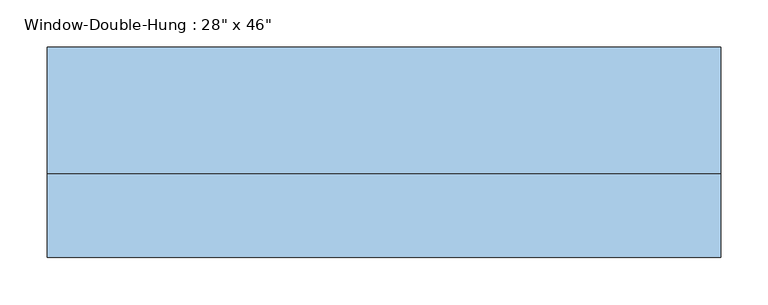
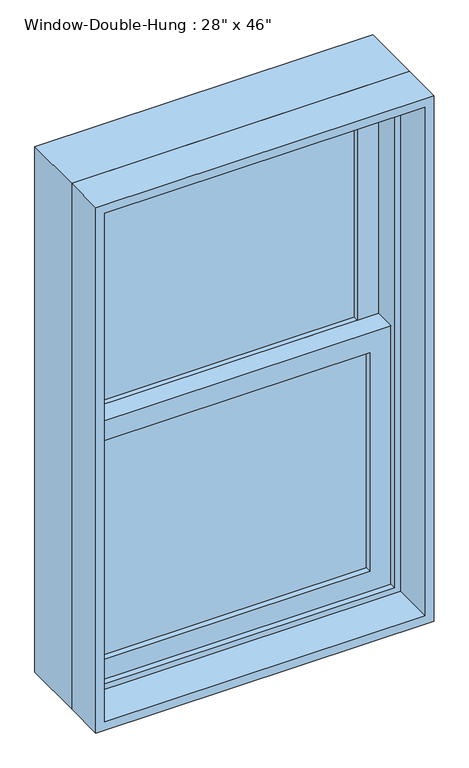
"""IFC4 building model written with IfcOpenShell, lengths in millimetres: window geometry."""

from ifc_helpers import new_model, si_unit, frame, origin, place, context, project, spatial, polyline, outline, extrude, source, transform, mapped, element, save


def window_4d695ea9(model_context):
    return source(origin(), model_context, "Body", "SweptSolid", [
        extrude(outline(polyline([(279.4, 31.75), (279.4, 25.4), (-279.4, 25.4), (-279.4, 31.75), (279.4, 31.75)])), frame((0.0, 0.0, 990.6), z_axis=(0.0, 0.0, 1.0), x_axis=(1.0, 0.0, 0.0)), (0.0, 0.0, 1.0), 485.775),
        extrude(outline(polyline([(-279.4, 19.05), (279.4, 19.05), (279.4, 12.7), (-279.4, 12.7), (-279.4, 19.05)])), frame((0.0, 0.0, 990.6), z_axis=(0.0, 0.0, 1.0), x_axis=(1.0, 0.0, 0.0)), (0.0, 0.0, 1.0), 485.775),
        extrude(outline(polyline([(279.4, 76.2), (279.4, 69.85), (-279.4, 69.85), (-279.4, 76.2), (279.4, 76.2)])), frame((0.0, 0.0, 1520.825), z_axis=(0.0, 0.0, 1.0), x_axis=(1.0, 0.0, 0.0)), (0.0, 0.0, 1.0), 485.775),
        extrude(outline(polyline([(-279.4, 63.5), (279.4, 63.5), (279.4, 57.15), (-279.4, 57.15), (-279.4, 63.5)])), frame((0.0, 0.0, 1520.825), z_axis=(0.0, 0.0, 1.0), x_axis=(1.0, 0.0, 0.0)), (0.0, 0.0, 1.0), 485.775),
        extrude(outline(polyline([(1520.825, -323.85), (946.15, -323.85), (946.15, 323.85), (1520.825, 323.85), (1520.825, -323.85)]), holes=[polyline([(1476.375, 279.4), (990.6, 279.4), (990.6, -279.4), (1476.375, -279.4), (1476.375, 279.4)])]), frame((0.0, 0.0, 0.0), z_axis=(0.0, 1.0, 0.0), x_axis=(0.0, 0.0, 1.0)), (0.0, 0.0, 1.0), 44.45),
        extrude(outline(polyline([(2051.05, -323.85), (1476.375, -323.85), (1476.375, 323.85), (2051.05, 323.85), (2051.05, -323.85)]), holes=[polyline([(2006.6, 279.4), (1520.825, 279.4), (1520.825, -279.4), (2006.6, -279.4), (2006.6, 279.4)])]), frame((0.0, 44.45, 0.0), z_axis=(0.0, 1.0, 0.0), x_axis=(0.0, 0.0, 1.0)), (0.0, 0.0, 1.0), 44.45),
        extrude(outline(polyline([(2082.8, -355.6), (914.4, -355.6), (914.4, 355.6), (2082.8, 355.6), (2082.8, -355.6)]), holes=[polyline([(2051.05, 323.85), (946.15, 323.85), (946.15, -323.85), (2051.05, -323.85), (2051.05, 323.85)])]), frame((0.0, -12.7, 0.0), z_axis=(0.0, 1.0, 0.0), x_axis=(0.0, 0.0, 1.0)), (0.0, 0.0, 1.0), 133.35),
        extrude(outline(polyline([(2082.8, 355.6), (2082.8, -355.6), (914.4, -355.6), (914.4, 355.6), (2082.8, 355.6)]), holes=[polyline([(2063.75, 336.55), (933.45, 336.55), (933.45, -336.55), (2063.75, -336.55), (2063.75, 336.55)])]), frame((0.0, -101.6, 0.0), z_axis=(0.0, 1.0, 0.0), x_axis=(0.0, 0.0, 1.0)), (0.0, 0.0, 1.0), 88.9),
    ])


if __name__ == "__main__":
    model = new_model("IFC4")
    model_context = context("Model", 3, world=origin())
    ifc_project = project(units=[si_unit("LENGTHUNIT", "METRE", prefix="MILLI")], contexts=[model_context])
    site = spatial("IfcSite", under=ifc_project)
    building = spatial("IfcBuilding", under=site)
    placement = place(None, origin())
    window_shape = window_4d695ea9(model_context)
    element("IfcWindow", 1, ObjectType="Window-Double-Hung : 28\" x 46\"", at=placement, inside=building, context=model_context, shape_type="MappedRepresentation", body=[
        mapped(window_shape, transform((0.0, 0.0, 0.0), x_axis=(1.0, 0.0, 0.0), y_axis=(0.0, 1.0, 0.0), z_axis=(0.0, 0.0, 1.0))),
    ])
    save(model, "model.ifc")

# Revit data of these elements
# Type "Window-Double-Hung : 28\" x 46\""
#   Type Mark = "12"
#   Fire Rating = "0.5h"
#   Construction Type Id = "DG-DR"
#   Assembly Code = "B2020100"
#   Analytic Construction = "Double glazing - domestic"
#   Wall Thickness [instance default] = 0' - 6"
#   Window Inset [instance default] = 0' - 0"
#   Visual Light Transmittance = 0.81
#   Thermal Resistance (R) = 1.8146 (h·ft²·°F)/BTU
#   Solar Heat Gain Coefficient = 0.76
#   Muntin Width = 1' - 10"
#   Muntin Height = 1' - 7 1/8"
#   Interior Wall Closure [instance default] = 0' - 1 1/2"
#   Rough Width = 2' - 4 1/2"
#   Rough Height = 3' - 10 1/2"
#   Frame Extension [instance default] = 0' - 1 1/4"
#   Exterior Wall Closure [instance default] = 0' - 0 1/2"
#   Extension Jamb [instance default] = 0' - 1 1/2"
#   Heat Transfer Coefficient (U) = 0.5511 BTU/(h·ft²·°F)
#   Height = 3' - 10"
#   Width = 2' - 4"
#   Define Thermal Properties by = 1
#   Top Muntin Visibility = yes
#   Indicator Visibility [instance default] = yes
#   Extension Jamb Visibility [instance default] = yes
#   Interior Trim Visibility [instance default] = yes
#   Exterior Trim Visibility [instance default] = yes
#   Define Thermal Properties by = 1
#   Bottom Muntin Visibility = yes
#   Muntin Pattern = Muntin Pattern_2x2 : Muntin Pattern_2x2
#   Interior Trim Material = Wood - Stained
#   Interior Trim = Trim-Window-Interior-Flat : Picture Frame
#   Exterior Trim Material = Clad - White
#   Exterior Trim = Trim-Window-Exterior-Flat : with Sill
#   Glass Panel Material = Glass
#   Exterior Frame Material = Clad - White
#   Interior Frame Material = Wood - Stained
#   Wall Closure = (empty or 0)
# Element 1 (IfcWindow, "Window-Double-Hung : 28\" x 46\"")
#   Wall Thickness = 0' - 8"
#   Extension Jamb = 0' - 3 1/2"
#   Materials on its faces: "Wood - Stained", "Glass", "Clad - White"
# Materials
#   "Wood - Stained": class "Wood", colour RGB 224 178 126, transparency 0, Cost = 0
#   "Clad - White": class "Wood", colour RGB 242 242 238, transparency 0, Cost = 0
#   "Glass": class "Glass", colour RGB 0 128 192, transparency 0.75, Description = "Soda Lime Glass", Cost = 0
